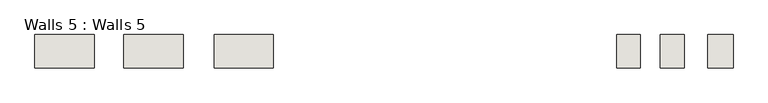
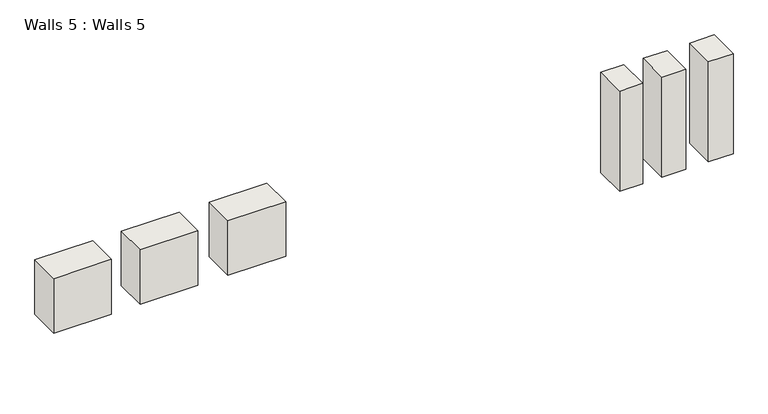
"""IFC4 building model written with IfcOpenShell, lengths in millimetres: wall geometry, Walls 5 : Walls 5."""

from ifc_helpers import new_model, si_unit, frame, origin, place, context, project, spatial, polyline, outline, extrude, source, transform, mapped, element, save


def walls_5_walls_5_e6219bd2(model_context):
    return source(origin(), model_context, "Body", "SweptSolid", [
        extrude(outline(polyline([(-2673.7815021, 3131.8919215), (-2978.5815021, 3131.8919215), (-2978.5815021, 3303.3419215), (-2673.7815021, 3303.3419215), (-2673.7815021, 3131.8919215)])), frame((0.0, 0.0, 7010.4), z_axis=(0.0, 0.0, 1.0), x_axis=(1.0, 0.0, 0.0)), (0.0, 0.0, 1.0), 304.8),
        extrude(outline(polyline([(-2216.5815021, 3131.8919215), (-2521.3815021, 3131.8919215), (-2521.3815021, 3303.3419215), (-2216.5815021, 3303.3419215), (-2216.5815021, 3131.8919215)])), frame((0.0, 0.0, 7010.4), z_axis=(0.0, 0.0, 1.0), x_axis=(1.0, 0.0, 0.0)), (0.0, 0.0, 1.0), 304.8),
        extrude(outline(polyline([(-1753.0315021, 3131.8919215), (-2057.8315021, 3131.8919215), (-2057.8315021, 3303.3419215), (-1753.0315021, 3303.3419215), (-1753.0315021, 3131.8919215)])), frame((0.0, 0.0, 7010.4), z_axis=(0.0, 0.0, 1.0), x_axis=(1.0, 0.0, 0.0)), (0.0, 0.0, 1.0), 304.8),
        extrude(outline(polyline([(131.9789298, 3131.8919215), (11.0429345, 3131.8919215), (11.0429345, 3303.3419215), (131.9789298, 3303.3419215), (131.9789298, 3131.8919215)])), frame((0.0, 0.0, 6756.4), z_axis=(0.0, 0.0, 1.0), x_axis=(1.0, 0.0, 0.0)), (0.0, 0.0, 1.0), 558.8),
        extrude(outline(polyline([(359.9381195, 3131.8919215), (234.3645239, 3131.8919215), (234.3645239, 3303.3419215), (359.9381195, 3303.3419215), (359.9381195, 3131.8919215)])), frame((0.0, 0.0, 6756.4), z_axis=(0.0, 0.0, 1.0), x_axis=(1.0, 0.0, 0.0)), (0.0, 0.0, 1.0), 558.8),
        extrude(outline(polyline([(609.8725099, 3131.8919215), (479.6613139, 3131.8919215), (479.6613139, 3303.3419215), (609.8725099, 3303.3419215), (609.8725099, 3131.8919215)])), frame((0.0, 0.0, 6756.4), z_axis=(0.0, 0.0, 1.0), x_axis=(1.0, 0.0, 0.0)), (0.0, 0.0, 1.0), 558.8),
    ])


if __name__ == "__main__":
    model = new_model("IFC4")
    model_context = context("Model", 3, world=origin())
    ifc_project = project(units=[si_unit("LENGTHUNIT", "METRE", prefix="MILLI")], contexts=[model_context])
    site = spatial("IfcSite", under=ifc_project)
    building = spatial("IfcBuilding", under=site)
    placement = place(None, origin())
    walls_5_walls_5_shape = walls_5_walls_5_e6219bd2(model_context)
    element("IfcWall", 1, ObjectType="Walls 5 : Walls 5", at=placement, inside=building, context=model_context, shape_type="MappedRepresentation", body=[
        mapped(walls_5_walls_5_shape, transform((0.0, 0.0, 0.0), x_axis=(1.0, 0.0, 0.0), y_axis=(0.0, 1.0, 0.0), z_axis=(0.0, 0.0, 1.0))),
    ])
    save(model, "model.ifc")

# Revit data of these elements
# Element 1 (IfcWall, "Walls 5 : Walls 5")
#   Materials on its faces: "Default Wall"
# Materials
#   "Default Wall": colour RGB 128 128 128, transparency 0
